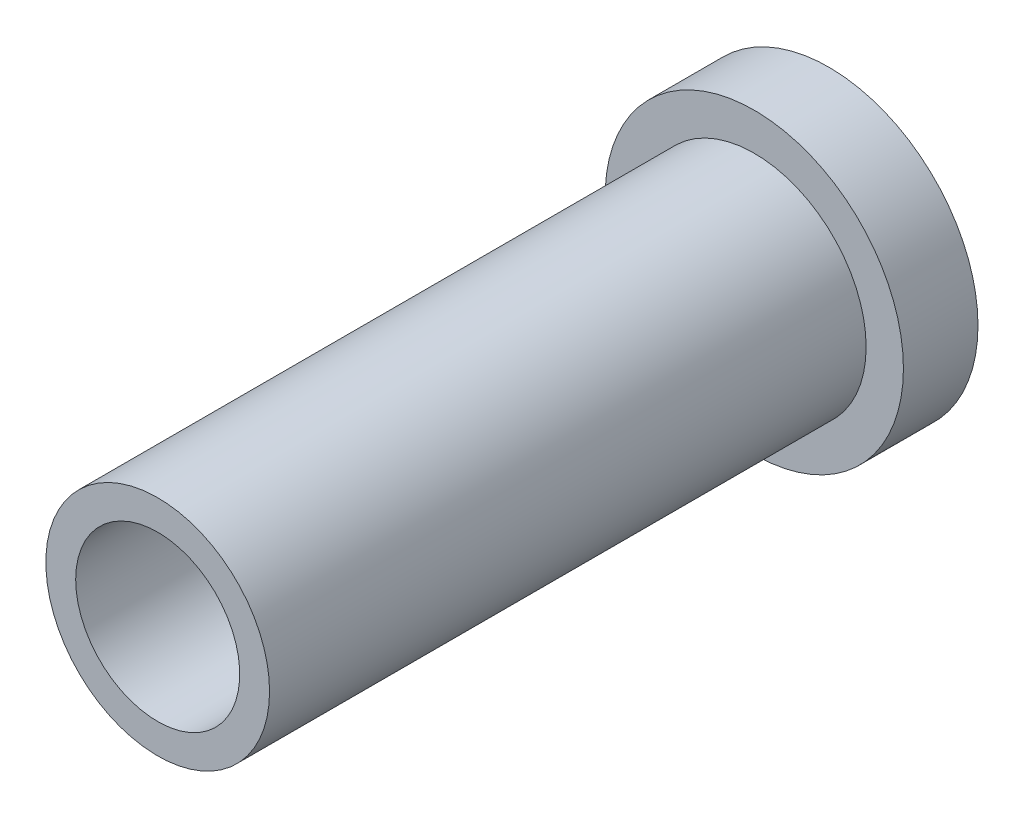
from build123d import *

# Parameters (mm, degrees)
FLANGE_PROFILE_20_R   = 10
FLANGE_20X5_DEPTH     = 5
SHANK_PROFILE_15_R    = 7.5
SHANK_15X40_DEPTH     = 40
BORE_PROFILE_11_R     = 5.5
BORE_11_THROUGH_DEPTH = 48.16990566


with BuildPart() as part:
    # Flange Profile Ø20 → Flange Ø20x5 (new body)
    with BuildSketch(Plane.XY):
        Circle(FLANGE_PROFILE_20_R)
    extrude(amount=FLANGE_20X5_DEPTH)

    # Shank Profile Ø15 → Shank Ø15x40 (add)
    with BuildSketch(Plane.XY.offset(5)):
        Circle(SHANK_PROFILE_15_R)
    extrude(amount=SHANK_15X40_DEPTH)

    # Bore Profile Ø11 → Bore Ø11 Through (cut, through all)
    with BuildSketch(Plane(origin=(0, 0, 0), x_dir=(-1, 0, 0), z_dir=(0, 0, -1))):
        Circle(BORE_PROFILE_11_R)
    extrude(amount=-BORE_11_THROUGH_DEPTH, mode=Mode.SUBTRACT)


solid = part.part
